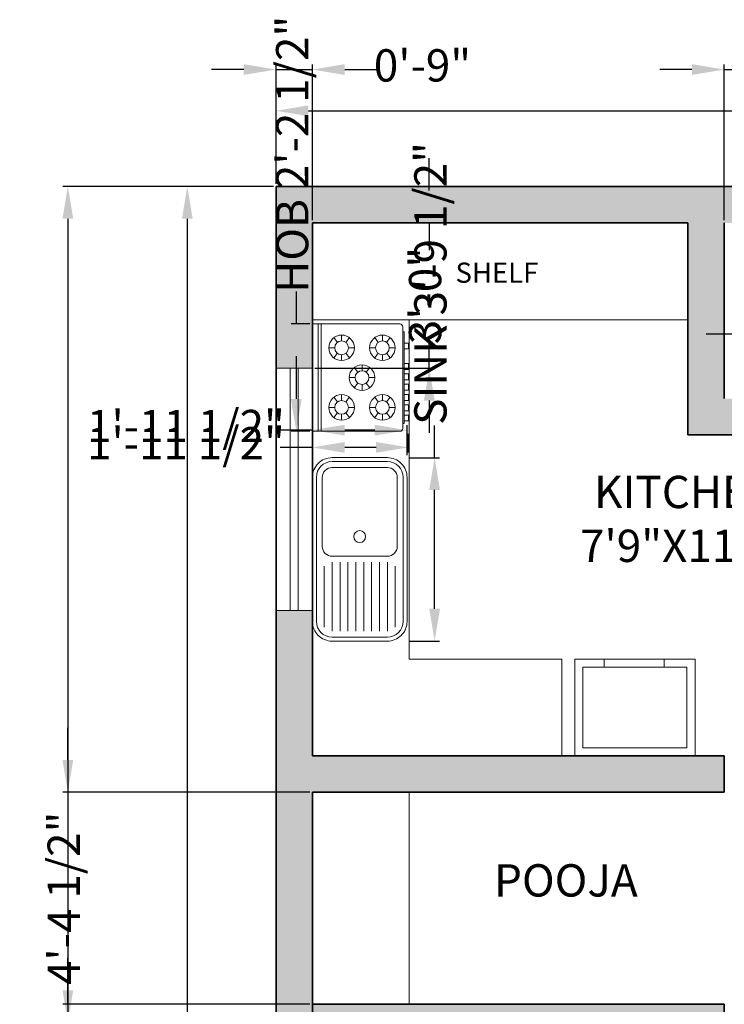
# Model space of a CAD drawing. Units: inches. Extents: x 2408 to 5087, y 2429 to 5085.
# Tile 10 of 12: x 2421 to 2595, y 2815 to 3058. Entities that reach past the tile are written whole.
import ezdxf

# ---------------------------------------------------------------- set-up
doc = ezdxf.new("R2010")
doc.units = ezdxf.units.IN
for name, color, linetype, lineweight in [('A-ANNO-DIMS', 2, 'Continuous', 18), ('A-ANNO-TEXT', 6, 'Continuous', 18), ('A-AREA-IDEN', 6, 'Continuous', 18), ('A-EQPM', 53, 'Continuous', 18), ('A-FLOR-CASE', 8, 'Continuous', 18), ('A-FLOR-FIXT', 9, 'Continuous', 18), ('A-GLAZ', 4, 'Continuous', 18), ('A-WALL', 7, 'Continuous', 35), ('A-WALL-PATT', 252, 'Continuous', 13)]:
    doc.layers.add(name, color=color, linetype=linetype, lineweight=lineweight)
doc.styles.get("Standard").update_dxf_attribs({"font": 'arial.ttf'})
doc.dimstyles.new('ISO-25', dxfattribs={"dimtxt": 8, "dimasz": 8, "dimexe": 1.25, "dimexo": 0.625, "dimtad": 0, "dimdec": 1, "dimlunit": 4, "dimtxsty": 'Standard', "dimcen": 2.5, "dimadec": 0, "dimazin": 0, "dimtfac": 1, "dimtdec": 1, "dimtmove": 0, "dimatfit": 3, "dimfxl": 1, "dimarcsym": 0})

# ---------------------------------------------------------------- blocks, each defined once
blk = doc.blocks.new('*D1')
at = {"layer": 'A-ANNO-DIMS', "color": 0, "lineweight": -2, "transparency": 16777216}
for p, q in [((2484.49, 3017.68), (2484.49, 3037.05)), ((2492.49, 3035.8), (2639.56, 3035.8)), ((2815.49, 3035.8), (2668.43, 3035.8)), ((2823.49, 3017.68), (2823.49, 3037.05))]:
    blk.add_line(p, q, dxfattribs=at)
at = {"layer": 'A-ANNO-DIMS', "color": 0, "transparency": 16777216}
for points in [[(2492.49, 3037.13), (2492.49, 3034.47), (2484.49, 3035.8)], [(2815.49, 3037.13), (2815.49, 3034.47), (2823.49, 3035.8)]]:
    blk.add_solid(points, dxfattribs=at)
at = {"layer": 'Defpoints', "color": 0, "transparency": 16777216}
for p in [(2823.49, 3035.8), (2484.49, 3017.05), (2823.49, 3017.05)]:
    blk.add_point(p, dxfattribs=at)
at = {"layer": 'A-ANNO-DIMS', "color": 0, "transparency": 16777216, "insert": (2653.99, 3035.8), "char_height": 8, "attachment_point": 5}
blk.add_mtext('28\'-3"', dxfattribs=at)
blk = doc.blocks.new('*D2')
at = {"layer": 'A-ANNO-DIMS', "color": 0, "lineweight": -2, "transparency": 16777216}
for p, q in [((2483.87, 3017.05), (2461.26, 3017.05)), ((2462.51, 3009.05), (2462.51, 2772.63)), ((2462.51, 2521.05), (2462.51, 2757.48)), ((2483.87, 2513.05), (2461.26, 2513.05))]:
    blk.add_line(p, q, dxfattribs=at)
at = {"layer": 'A-ANNO-DIMS', "color": 0, "transparency": 16777216}
for points in [[(2461.17, 3009.05), (2463.84, 3009.05), (2462.51, 3017.05)], [(2461.17, 2521.05), (2463.84, 2521.05), (2462.51, 2513.05)]]:
    blk.add_solid(points, dxfattribs=at)
at = {"layer": 'Defpoints', "color": 0, "transparency": 16777216}
for p in [(2484.49, 3017.05), (2462.51, 2513.05), (2484.49, 2513.05)]:
    blk.add_point(p, dxfattribs=at)
at = {"layer": 'A-ANNO-DIMS', "color": 0, "transparency": 16777216, "insert": (2462.51, 2765.05), "char_height": 8, "attachment_point": 5, "rotation": 90}
blk.add_mtext("42'", dxfattribs=at)
blk = doc.blocks.new('g')
for p, q in [((2588.75, 3095.5), (2617.52, 3095.5)), ((2588.75, 3095.5), (2588.75, 3072.07)), ((2617.52, 3095.5), (2617.52, 3072.07)), ((2588.75, 3093.93), (2617.52, 3093.93)), ((2588.75, 3093.14), (2617.52, 3093.14)), ((2593.68, 3088.79), (2592.42, 3089.75)), ((2595.15, 3091.1), (2595.15, 3089.52)), ((2596.62, 3088.79), (2597.87, 3089.75)), ((2609.65, 3088.79), (2608.4, 3089.75)), ((2611.12, 3091.1), (2611.12, 3089.52)), ((2612.59, 3088.79), (2613.85, 3089.75)), ((2593.3, 3087.68), (2591.72, 3087.68)), ((2598.57, 3087.68), (2596.99, 3087.68)), ((2607.7, 3087.68), (2609.28, 3087.68)), ((2612.97, 3087.68), (2614.55, 3087.68)), ((2592.42, 3085.61), (2593.68, 3086.56)), ((2595.15, 3085.83), (2595.15, 3084.25)), ((2597.87, 3085.61), (2596.62, 3086.56)), ((2601.66, 3083.33), (2600.41, 3084.28)), ((2603.14, 3085.64), (2603.14, 3084.06)), ((2604.61, 3083.33), (2605.86, 3084.28)), ((2608.4, 3085.61), (2609.65, 3086.56)), ((2611.12, 3085.83), (2611.12, 3084.25)), ((2613.85, 3085.61), (2612.59, 3086.56)), ((2601.29, 3082.21), (2599.71, 3082.21)), ((2606.56, 3082.21), (2604.98, 3082.21)), ((2592.42, 3078.82), (2593.68, 3077.87)), ((2595.15, 3078.6), (2595.15, 3080.17)), ((2597.87, 3078.82), (2596.62, 3077.87)), ((2600.41, 3080.14), (2601.66, 3081.09)), ((2603.14, 3080.36), (2603.14, 3078.79)), ((2605.86, 3080.14), (2604.61, 3081.09)), ((2608.4, 3078.82), (2609.65, 3077.87)), ((2611.12, 3078.6), (2611.12, 3080.17)), ((2613.85, 3078.82), (2612.59, 3077.87)), ((2593.3, 3076.75), (2591.72, 3076.75)), ((2598.57, 3076.75), (2596.99, 3076.75)), ((2607.7, 3076.75), (2609.28, 3076.75)), ((2612.97, 3076.75), (2614.55, 3076.75)), ((2593.68, 3075.63), (2592.42, 3074.68)), ((2595.15, 3073.33), (2595.15, 3074.9)), ((2596.62, 3075.63), (2597.87, 3074.68)), ((2609.65, 3075.63), (2608.4, 3074.68)), ((2611.12, 3073.33), (2611.12, 3074.9)), ((2612.59, 3075.63), (2613.85, 3074.68)), ((2589.54, 3071.29), (2616.73, 3071.29)), ((2590.84, 3070.89), (2590.84, 3071.29)), ((2590.84, 3070.89), (2615.43, 3070.89)), ((2591.53, 3070.89), (2591.53, 3069.8)), ((2593.12, 3069.8), (2593.12, 3070.89)), ((2594.28, 3070.89), (2594.28, 3069.8)), ((2595.88, 3069.8), (2595.88, 3070.89)), ((2597.04, 3070.89), (2597.04, 3069.8)), ((2598.63, 3069.8), (2598.63, 3070.89)), ((2599.79, 3070.89), (2599.79, 3069.8)), ((2601.39, 3069.8), (2601.39, 3070.89)), ((2602.55, 3070.89), (2602.55, 3069.8)), ((2604.14, 3069.8), (2604.14, 3070.89)), ((2605.31, 3070.89), (2605.31, 3069.8)), ((2606.9, 3069.8), (2606.9, 3070.89)), ((2610.82, 3070.89), (2610.82, 3069.8)), ((2612.41, 3069.8), (2612.41, 3070.89)), ((2615.43, 3070.89), (2615.43, 3071.29)), ((2591.53, 3069.8), (2593.12, 3069.8)), ((2594.28, 3069.8), (2595.88, 3069.8)), ((2597.04, 3069.8), (2598.63, 3069.8)), ((2599.79, 3069.8), (2601.39, 3069.8)), ((2602.55, 3069.8), (2604.14, 3069.8)), ((2605.31, 3069.8), (2606.9, 3069.8)), ((2610.82, 3069.8), (2612.41, 3069.8))]:
    blk.add_line(p, q)
for centre, radius in [((2595.15, 3087.68), 3.42), ((2595.15, 3087.68), 1.85), ((2611.12, 3087.68), 3.42), ((2611.12, 3087.68), 1.85), ((2603.14, 3082.21), 3.42), ((2603.14, 3082.21), 1.85), ((2595.15, 3076.75), 3.42), ((2611.12, 3076.75), 3.42), ((2595.15, 3076.75), 1.85), ((2611.12, 3076.75), 1.85)]:
    blk.add_circle(centre, radius)
for centre, start, end in [((2589.54, 3072.07), 180, 270), ((2616.73, 3072.07), 270, 0)]:
    blk.add_arc(centre, 0.787, start, end)
blk = doc.blocks.new('sink')
for p, q in [((2402.653, 2953.482), (2405.527, 2953.482)), ((2402.535, 2953.325), (2403.755, 2953.325)), ((2402.338, 2952.065), (2402.338, 2953.167)), ((2402.456, 2953.167), (2403.834, 2953.167)), ((2405.842, 2953.167), (2405.842, 2952.065)), ((2402.456, 2953.01), (2403.834, 2953.01)), ((2402.456, 2952.852), (2403.834, 2952.852)), ((2402.456, 2952.695), (2403.834, 2952.695)), ((2402.456, 2952.537), (2403.834, 2952.537)), ((2402.456, 2952.38), (2403.834, 2952.38)), ((2402.456, 2952.222), (2403.834, 2952.222)), ((2402.456, 2952.065), (2403.834, 2952.065)), ((2402.535, 2951.907), (2403.755, 2951.907)), ((2405.527, 2951.75), (2402.653, 2951.75))]:
    blk.add_line(p, q)
at = {"flags": 128}
for points in [[(2405.527, 2953.561, -0.414214), (2405.921, 2953.167), (2405.921, 2952.065, -0.414214), (2405.527, 2951.671), (2402.653, 2951.671, -0.414214), (2402.259, 2952.065), (2402.259, 2953.167, -0.414214), (2402.653, 2953.561)], [(2405.527, 2953.364, -0.414214), (2405.724, 2953.167), (2405.724, 2952.065, -0.414214), (2405.527, 2951.868), (2404.149, 2951.868, -0.414214), (2403.952, 2952.065), (2403.952, 2953.167, -0.414214), (2404.149, 2953.364)]]:
    blk.add_lwpolyline(points, format="xyb", close=True, dxfattribs=at)
blk.add_circle((2404.346, 2952.616), 0.118)
for centre, start, end in [((2402.653, 2953.167), 90, 180), ((2405.527, 2953.167), 0, 90), ((2402.653, 2952.065), 180, 270), ((2405.527, 2952.065), 270, 0)]:
    blk.add_arc(centre, 0.315, start, end)
blk = doc.blocks.new('WIN-60x9')
for p, q in [((3.5, 60), (3.5, 0)), ((5.5, 60), (5.5, 0))]:
    blk.add_line(p, q)
blk.add_lwpolyline([(0, 60), (9, 60), (9, 0), (0, 0)], close=True)
blk = doc.blocks.new('*D48')
at = {"layer": 'A-ANNO-DIMS', "color": 0, "lineweight": -2, "transparency": 16777216}
for p, q in [((2607, 2983.48), (2607, 2979.26)), ((2619.98, 2983.48), (2619.98, 2979.26)), ((2599, 2980.51), (2591, 2980.51)), ((2607, 2980.51), (2619.98, 2980.51)), ((2627.98, 2980.51), (2635.98, 2980.51))]:
    blk.add_line(p, q, dxfattribs=at)
at = {"layer": 'A-ANNO-DIMS', "color": 0, "transparency": 16777216}
for points in [[(2599, 2981.84), (2599, 2979.18), (2607, 2980.51)], [(2627.98, 2981.84), (2627.98, 2979.18), (2619.98, 2980.51)]]:
    blk.add_solid(points, dxfattribs=at)
at = {"layer": 'Defpoints', "color": 0, "transparency": 16777216}
for p in [(2607, 2984.1), (2619.98, 2984.1), (2619.98, 2980.51)]:
    blk.add_point(p, dxfattribs=at)
at = {"layer": 'A-ANNO-DIMS', "color": 0, "transparency": 16777216, "insert": (2660.61, 2980.51), "char_height": 8, "attachment_point": 5}
blk.add_mtext('1\'-1" TYP.', dxfattribs=at)
blk = doc.blocks.new('*D55')
at = {"layer": 'A-ANNO-DIMS', "color": 0, "lineweight": -2, "transparency": 16777216}
for p, q in [((2489.51, 2983.02), (2489.51, 2991.02)), ((2492.87, 2983.02), (2488.26, 2983.02)), ((2489.51, 2964.44), (2489.51, 2975.02)), ((2492.87, 2956.44), (2488.26, 2956.44))]:
    blk.add_line(p, q, dxfattribs=at)
at = {"layer": 'A-ANNO-DIMS', "color": 0, "transparency": 16777216}
for points in [[(2488.17, 2975.02), (2490.84, 2975.02), (2489.51, 2983.02)], [(2488.17, 2964.44), (2490.84, 2964.44), (2489.51, 2956.44)]]:
    blk.add_solid(points, dxfattribs=at)
at = {"layer": 'Defpoints', "color": 0, "transparency": 16777216}
for p in [(2489.51, 2983.02), (2493.49, 2983.02), (2493.49, 2956.44)]:
    blk.add_point(p, dxfattribs=at)
at = {"layer": 'A-ANNO-DIMS', "color": 0, "transparency": 16777216, "insert": (2489.51, 3025.04), "char_height": 8, "attachment_point": 5, "rotation": 90}
blk.add_mtext('HOB 2\'-2 1/2"', dxfattribs=at)
blk = doc.blocks.new('*D56')
at = {"layer": 'A-ANNO-DIMS', "color": 0, "lineweight": -2, "transparency": 16777216}
for p, q in [((2493.49, 2955.81), (2493.49, 2951.2)), ((2517.24, 2955.81), (2517.24, 2951.2)), ((2493.49, 2952.45), (2485.49, 2952.45)), ((2509.24, 2952.45), (2501.49, 2952.45))]:
    blk.add_line(p, q, dxfattribs=at)
at = {"layer": 'A-ANNO-DIMS', "color": 0, "transparency": 16777216}
for points in [[(2501.49, 2953.78), (2501.49, 2951.12), (2493.49, 2952.45)], [(2509.24, 2953.78), (2509.24, 2951.12), (2517.24, 2952.45)]]:
    blk.add_solid(points, dxfattribs=at)
at = {"layer": 'Defpoints', "color": 0, "transparency": 16777216}
for p in [(2493.49, 2956.44), (2517.24, 2956.44), (2493.49, 2952.45)]:
    blk.add_point(p, dxfattribs=at)
at = {"layer": 'A-ANNO-DIMS', "color": 0, "transparency": 16777216, "insert": (2462.18, 2952.45), "char_height": 8, "attachment_point": 5}
blk.add_mtext('1\'-11 1/2"', dxfattribs=at)
blk = doc.blocks.new('*D57')
at = {"layer": 'A-ANNO-DIMS', "color": 0, "lineweight": -2, "transparency": 16777216}
for p, q in [((2523.75, 2949.9), (2523.75, 2957.9)), ((2517.56, 2949.9), (2525, 2949.9)), ((2523.75, 2912.48), (2523.75, 2941.9)), ((2517.56, 2904.48), (2525, 2904.48))]:
    blk.add_line(p, q, dxfattribs=at)
at = {"layer": 'A-ANNO-DIMS', "color": 0, "transparency": 16777216}
for points in [[(2522.42, 2941.9), (2525.08, 2941.9), (2523.75, 2949.9)], [(2522.42, 2912.48), (2525.08, 2912.48), (2523.75, 2904.48)]]:
    blk.add_solid(points, dxfattribs=at)
at = {"layer": 'Defpoints', "color": 0, "transparency": 16777216}
for p in [(2516.94, 2949.9), (2523.75, 2949.9), (2516.94, 2904.48)]:
    blk.add_point(p, dxfattribs=at)
at = {"layer": 'A-ANNO-DIMS', "color": 0, "transparency": 16777216, "insert": (2523.75, 2993.05), "char_height": 8, "attachment_point": 5, "rotation": 90}
blk.add_mtext('SINK 3\'-9 1/2"', dxfattribs=at)
blk = doc.blocks.new('*D58')
at = {"layer": 'A-ANNO-DIMS', "color": 0, "lineweight": -2, "transparency": 16777216}
for p, q in [((2493.49, 2950.53), (2493.49, 2957.96)), ((2516.94, 2950.53), (2516.94, 2957.96)), ((2493.49, 2956.71), (2485.49, 2956.71)), ((2508.94, 2956.71), (2501.49, 2956.71))]:
    blk.add_line(p, q, dxfattribs=at)
at = {"layer": 'A-ANNO-DIMS', "color": 0, "transparency": 16777216}
for points in [[(2501.49, 2958.05), (2501.49, 2955.38), (2493.49, 2956.71)], [(2508.94, 2958.05), (2508.94, 2955.38), (2516.94, 2956.71)]]:
    blk.add_solid(points, dxfattribs=at)
at = {"layer": 'Defpoints', "color": 0, "transparency": 16777216}
for p in [(2493.49, 2956.71), (2493.49, 2949.9), (2516.94, 2949.9)]:
    blk.add_point(p, dxfattribs=at)
at = {"layer": 'A-ANNO-DIMS', "color": 0, "transparency": 16777216, "insert": (2462.18, 2956.71), "char_height": 8, "attachment_point": 5}
blk.add_mtext('1\'-11 1/2"', dxfattribs=at)
blk = doc.blocks.new('*D62')
at = {"layer": 'A-ANNO-DIMS', "color": 0, "lineweight": -2, "transparency": 16777216}
for p, q in [((2432.93, 2875.05), (2432.93, 2883.05)), ((2492.87, 2867.05), (2431.68, 2867.05)), ((2432.93, 2867.05), (2432.93, 2861.54)), ((2432.93, 2814.55), (2432.93, 2820.06)), ((2492.87, 2814.55), (2431.68, 2814.55)), ((2432.93, 2806.55), (2432.93, 2798.55))]:
    blk.add_line(p, q, dxfattribs=at)
at = {"layer": 'A-ANNO-DIMS', "color": 0, "transparency": 16777216}
for points in [[(2431.59, 2875.05), (2434.26, 2875.05), (2432.93, 2867.05)], [(2431.59, 2806.55), (2434.26, 2806.55), (2432.93, 2814.55)]]:
    blk.add_solid(points, dxfattribs=at)
at = {"layer": 'Defpoints', "color": 0, "transparency": 16777216}
for p in [(2432.93, 2867.05), (2493.49, 2867.05), (2493.49, 2814.55)]:
    blk.add_point(p, dxfattribs=at)
at = {"layer": 'A-ANNO-DIMS', "color": 0, "transparency": 16777216, "insert": (2432.93, 2840.8), "char_height": 8, "attachment_point": 5, "rotation": 90}
blk.add_mtext('4\'-4 1/2"', dxfattribs=at)
blk = doc.blocks.new('*D63')
at = {"layer": 'A-ANNO-DIMS', "color": 0, "lineweight": -2, "transparency": 16777216}
for p, q in [((2476.49, 3046), (2468.49, 3046)), ((2484.49, 3017.68), (2484.49, 3047.25)), ((2484.49, 3046), (2493.49, 3046)), ((2493.49, 3008.68), (2493.49, 3047.25)), ((2501.49, 3046), (2509.49, 3046))]:
    blk.add_line(p, q, dxfattribs=at)
at = {"layer": 'A-ANNO-DIMS', "color": 0, "transparency": 16777216}
for points in [[(2476.49, 3047.34), (2476.49, 3044.67), (2484.49, 3046)], [(2501.49, 3047.34), (2501.49, 3044.67), (2493.49, 3046)]]:
    blk.add_solid(points, dxfattribs=at)
at = {"layer": 'Defpoints', "color": 0, "transparency": 16777216}
for p in [(2493.49, 3046), (2484.49, 3017.05), (2493.49, 3008.05)]:
    blk.add_point(p, dxfattribs=at)
at = {"layer": 'A-ANNO-DIMS', "color": 0, "transparency": 16777216, "insert": (2520.75, 3046), "char_height": 8, "attachment_point": 5}
blk.add_mtext('0\'-9"', dxfattribs=at)
blk = doc.blocks.new('*D66')
at = {"layer": 'A-ANNO-DIMS', "color": 0, "lineweight": -2, "transparency": 16777216}
for p, q in [((2483.87, 3017.05), (2431.68, 3017.05)), ((2432.93, 3009.05), (2432.93, 2767.25)), ((2432.93, 2477.75), (2432.93, 2719.56)), ((2461.25, 2469.75), (2431.68, 2469.75))]:
    blk.add_line(p, q, dxfattribs=at)
at = {"layer": 'A-ANNO-DIMS', "color": 0, "transparency": 16777216}
for points in [[(2431.59, 3009.05), (2434.26, 3009.05), (2432.93, 3017.05)], [(2431.59, 2477.75), (2434.26, 2477.75), (2432.93, 2469.75)]]:
    blk.add_solid(points, dxfattribs=at)
at = {"layer": 'Defpoints', "color": 0, "transparency": 16777216}
for p in [(2432.93, 3017.05), (2484.49, 3017.05), (2461.88, 2469.75)]:
    blk.add_point(p, dxfattribs=at)
at = {"layer": 'A-ANNO-DIMS', "color": 0, "transparency": 16777216, "insert": (2432.93, 2743.4), "char_height": 8, "attachment_point": 5, "rotation": 90}
blk.add_mtext('45\'-7 1/2"', dxfattribs=at)
blk = doc.blocks.new('*D70')
at = {"layer": 'A-ANNO-DIMS', "color": 0, "lineweight": -2, "transparency": 16777216}
for p, q in [((2587.49, 3046), (2579.49, 3046)), ((2595.49, 3008.68), (2595.49, 3047.25)), ((2595.49, 3046), (2601.49, 3046)), ((2601.49, 3008.68), (2601.49, 3047.25)), ((2609.49, 3046), (2617.49, 3046))]:
    blk.add_line(p, q, dxfattribs=at)
at = {"layer": 'A-ANNO-DIMS', "color": 0, "transparency": 16777216}
for points in [[(2587.49, 3047.34), (2587.49, 3044.67), (2595.49, 3046)], [(2609.49, 3047.34), (2609.49, 3044.67), (2601.49, 3046)]]:
    blk.add_solid(points, dxfattribs=at)
at = {"layer": 'Defpoints', "color": 0, "transparency": 16777216}
for p in [(2601.49, 3046), (2595.49, 3008.05), (2601.49, 3008.05)]:
    blk.add_point(p, dxfattribs=at)
at = {"layer": 'A-ANNO-DIMS', "color": 0, "transparency": 16777216, "insert": (2628.75, 3046), "char_height": 8, "attachment_point": 5}
blk.add_mtext('0\'-6"', dxfattribs=at)
blk = doc.blocks.new('*D72')
at = {"layer": 'A-ANNO-DIMS', "color": 0, "lineweight": -2, "transparency": 16777216}
for p, q in [((2522.44, 3016.05), (2522.44, 3024.05)), ((2494.12, 3008.05), (2523.69, 3008.05)), ((2522.44, 3008.05), (2522.44, 3001.31)), ((2522.44, 2972.05), (2522.44, 2978.8)), ((2494.12, 2972.05), (2523.69, 2972.05)), ((2522.44, 2964.05), (2522.44, 2956.05))]:
    blk.add_line(p, q, dxfattribs=at)
at = {"layer": 'A-ANNO-DIMS', "color": 0, "transparency": 16777216}
for points in [[(2521.11, 3016.05), (2523.78, 3016.05), (2522.44, 3008.05)], [(2521.11, 2964.05), (2523.78, 2964.05), (2522.44, 2972.05)]]:
    blk.add_solid(points, dxfattribs=at)
at = {"layer": 'Defpoints', "color": 0, "transparency": 16777216}
for p in [(2493.49, 3008.05), (2493.49, 2972.05), (2522.44, 2972.05)]:
    blk.add_point(p, dxfattribs=at)
at = {"layer": 'A-ANNO-DIMS', "color": 0, "transparency": 16777216, "insert": (2522.44, 2990.05), "char_height": 8, "attachment_point": 5, "rotation": 90}
blk.add_mtext('3\'-0"', dxfattribs=at)
blk = doc.blocks.new('*D79')
at = {"layer": 'A-ANNO-DIMS', "color": 0, "lineweight": -2, "transparency": 16777216}
for p, q in [((2432.93, 2818.05), (2432.93, 2826.05)), ((2693.87, 2810.05), (2431.68, 2810.05)), ((2432.93, 2810.05), (2432.93, 2809.38)), ((2432.93, 2786.05), (2432.93, 2786.73)), ((2693.87, 2786.05), (2431.68, 2786.05)), ((2432.93, 2778.05), (2432.93, 2770.05))]:
    blk.add_line(p, q, dxfattribs=at)
at = {"layer": 'A-ANNO-DIMS', "color": 0, "transparency": 16777216}
for points in [[(2431.59, 2818.05), (2434.26, 2818.05), (2432.93, 2810.05)], [(2431.59, 2778.05), (2434.26, 2778.05), (2432.93, 2786.05)]]:
    blk.add_solid(points, dxfattribs=at)
at = {"layer": 'Defpoints', "color": 0, "transparency": 16777216}
for p in [(2432.93, 2810.05), (2694.49, 2810.05), (2694.49, 2786.05)]:
    blk.add_point(p, dxfattribs=at)
at = {"layer": 'A-ANNO-DIMS', "color": 0, "transparency": 16777216, "insert": (2432.93, 2798.05), "char_height": 8, "attachment_point": 5, "rotation": 90}
blk.add_mtext('2\'-0"', dxfattribs=at)

msp = doc.modelspace()

# ---------------------------------------------------------------- hatches: boundary and pattern name
at = {"layer": 'A-WALL-PATT'}
h = msp.add_hatch(color=256, dxfattribs=at)
h.dxf.hatch_style = 1
h.paths.add_polyline_path([(2493.49, 2613.55), (2523.49, 2613.55), (2523.49, 2622.55), (2493.49, 2622.55), (2493.49, 2714.8), (2484.49, 2714.8), (2484.49, 2497.75), (2493.49, 2497.75)])
h.paths.add_polyline_path([(2613.49, 2615.42), (2613.49, 2622.55), (2583.49, 2622.55), (2583.49, 2613.55), (2613.46, 2613.55, -0.009707)])
h.paths.add_polyline_path([(2823.49, 2634.55), (2814.49, 2634.55), (2814.49, 2622.55), (2694.49, 2622.55), (2694.49, 2670.55), (2706.49, 2670.55), (2706.49, 2675.05), (2694.49, 2675.05), (2694.49, 2750.05), (2685.49, 2750.05), (2685.49, 2622.55), (2661.49, 2622.55), (2661.49, 2613.55), (2814.49, 2613.55), (2814.49, 2522.05), (2688.49, 2522.05), (2688.49, 2513.05), (2823.49, 2513.05)])
h.paths.add_polyline_path([(2823.49, 2837.05), (2814.49, 2837.05), (2814.49, 2819.05), (2685.49, 2819.05), (2685.49, 2786.05), (2694.49, 2786.05), (2694.49, 2810.05), (2814.49, 2810.05), (2814.49, 2772.55), (2823.49, 2772.55)])
h.paths.add_polyline_path([(2694.49, 2964.55), (2595.49, 2964.55), (2595.49, 3008.05), (2601.49, 3008.05), (2601.49, 3017.05), (2484.49, 3017.05), (2484.49, 2972.05), (2493.49, 2972.05), (2493.49, 3008.05), (2586.49, 3008.05), (2586.49, 2955.55), (2685.49, 2955.55), (2685.49, 2854.87), (2694.49, 2854.87)])
h.paths.add_polyline_path([(2493.49, 2867.05), (2595.49, 2867.05), (2595.49, 2876.05), (2493.49, 2876.05), (2493.49, 2912.05), (2484.49, 2912.05), (2484.49, 2774.8), (2493.49, 2774.8)])
h.paths.add_polyline_path([(2595.49, 2814.55), (2493.49, 2814.55), (2493.49, 2810.05), (2595.49, 2810.05)], flags=17)
h.paths.add_polyline_path([(2724.49, 3017.05), (2625.49, 3017.05), (2625.49, 3008.05), (2685.49, 3008.05), (2685.49, 2994.55), (2694.49, 2994.55), (2694.49, 3008.05), (2724.49, 3008.05)])
h.paths.add_polyline_path([(2823.49, 3017.05), (2784.49, 3017.05), (2784.49, 3008.05), (2814.49, 3008.05), (2814.49, 2913.55), (2814.56, 2897.05), (2823.49, 2897.05)])
h.paths.add_polyline_path([(2823.49, 2712.55), (2814.61, 2712.55), (2814.66, 2701.27), (2814.49, 2701.27), (2814.49, 2675.05), (2740.99, 2675.05), (2740.99, 2687.05), (2736.49, 2687.05), (2736.49, 2670.55), (2814.49, 2670.55), (2814.49, 2658.55), (2823.49, 2658.55)], flags=17)

# ---------------------------------------------------------------- linework, layer by layer
at = {"layer": 'A-EQPM'}
for p, q in [((2588.25, 2900.05), (2558.48, 2900.05)), ((2565.77, 2898.05), (2565.77, 2900.05)), ((2580.63, 2898.05), (2580.63, 2900.05)), ((2588.25, 2900.05), (2588.25, 2876.05))]:
    msp.add_line(p, q, dxfattribs=at)
for points in [[(2588.25, 2876.05), (2558.48, 2876.05), (2558.48, 2900.05), (2588.25, 2900.05)], [(2586.25, 2878.05), (2560.48, 2878.05), (2560.48, 2898.05), (2586.25, 2898.05)]]:
    msp.add_lwpolyline(points, close=True, dxfattribs=at)
at = {"layer": 'A-FLOR-CASE'}
for p, q in [((2586.49, 2984.05), (2493.49, 2984.05)), ((2517.49, 2984.05), (2517.49, 2900.05)), ((2555.29, 2900.05), (2517.49, 2900.05)), ((2555.29, 2900.05), (2555.29, 2876.05)), ((2517.49, 2867.05), (2517.49, 2814.55))]:
    msp.add_line(p, q, dxfattribs=at)
at = {"layer": 'A-WALL'}
for p, q in [((2823.49, 3017.05), (2484.49, 3017.05)), ((2484.49, 3017.05), (2484.49, 2497.75)), ((2493.49, 3008.05), (2493.49, 2876.05)), ((2586.49, 3008.05), (2493.49, 3008.05)), ((2586.49, 3008.05), (2586.49, 2955.55)), ((2595.49, 3008.05), (2595.49, 2964.55)), ((2685.49, 2955.55), (2586.49, 2955.55)), ((2595.49, 2876.05), (2493.49, 2876.05)), ((2595.49, 2876.05), (2595.49, 2867.05)), ((2595.49, 2867.05), (2493.49, 2867.05)), ((2493.49, 2867.05), (2493.49, 2622.55)), ((2595.49, 2814.55), (2493.49, 2814.55)), ((2595.49, 2814.55), (2595.49, 2810.05))]:
    msp.add_line(p, q, dxfattribs=at)

# ---------------------------------------------------------------- block references
at = {"layer": 'A-EQPM', "xscale": 0.9241143459422847, "yscale": 0.9241143459422847, "zscale": 0.9241143459422847, "rotation": 90}
msp.add_blockref('g', (5354.09, 564.13), dxfattribs=at)
at = {"layer": 'A-FLOR-FIXT', "xscale": 12.40512744421288, "yscale": 12.40512744421288, "zscale": 12.40512744421288, "rotation": 90}
msp.add_blockref('sink', (39132.79, -26895.85), dxfattribs=at)
at = {"layer": 'A-GLAZ'}
msp.add_blockref('WIN-60x9', (2484.49, 2912.05), dxfattribs=at)

# ---------------------------------------------------------------- texts
at = {"layer": 'A-ANNO-TEXT', "insert": (2487.74, 2998.21), "char_height": 5, "attachment_point": 1}
msp.add_mtext_dynamic_manual_height_columns('\\pxqc;SHELF', width=102.8772, gutter_width=12.5, heights=[0], dxfattribs=at)
at = {"layer": 'A-AREA-IDEN', "char_height": 8, "attachment_point": 1}
for s, insert in [('\\pxqc;KITCHEN\\P7\'9"X11\'0"', (2534.8, 2945.41)), ('\\pxqc;POOJA', (2504.82, 2849.24))]:
    msp.add_mtext_dynamic_manual_height_columns(s, width=102.8772, gutter_width=12.5, heights=[0], dxfattribs=dict(at, insert=insert))

# ---------------------------------------------------------------- dimensions: what is measured, and where the dimension line sits
at = {"layer": 'A-ANNO-DIMS'}
for base, p1, p2, text, picture, middle in [((2489.51, 2983.02), (2493.49, 2956.44), (2493.49, 2983.02), 'HOB <>', '*D55', (2489.51, 3025.04)), ((2523.75, 2949.9), (2516.94, 2904.48), (2516.94, 2949.9), 'SINK <>', '*D57', (2523.75, 2993.05))]:
    dim = msp.add_linear_dim(base=base, p1=p1, p2=p2, angle=90, text=text, dimstyle='ISO-25', override={"dimdec": 1, "dimlfac": 1, "dimrnd": 0, "dimzin": 1, "dimdsep": 46, "dimlunit": 4, "dimfrac": 2}, dxfattribs=at)
    dim.commit()
    dim.dimension.update_dxf_attribs({"geometry": picture, "text_midpoint": middle})
for base, p1, p2, override, picture, middle in [((2493.49, 3046), (2484.49, 3017.05), (2493.49, 3008.05), {"dimdec": 1, "dimlfac": 1, "dimrnd": 0, "dimzin": 1, "dimdsep": 46, "dimlunit": 4, "dimfrac": 2}, '*D63', (2520.75, 3046)), ((2601.49, 3046), (2595.49, 3008.05), (2601.49, 3008.05), {"dimdec": 1, "dimlfac": 1, "dimrnd": 0, "dimzin": 1, "dimdsep": 46, "dimlunit": 4, "dimfrac": 2}, '*D70', (2628.75, 3046)), ((2823.49, 3035.8), (2484.49, 3017.05), (2823.49, 3017.05), {"dimclrd": 0, "dimclre": 0, "dimclrt": 0}, '*D1', (2653.99, 3035.8))]:
    dim = msp.add_linear_dim(base=base, p1=p1, p2=p2, dimstyle='ISO-25', override=override, dxfattribs=at)
    dim.commit()
    dim.dimension.update_dxf_attribs({"geometry": picture, "text_midpoint": middle})
for base, p1, p2, angle, override, picture, middle in [((2522.44, 2972.05), (2493.49, 3008.05), (2493.49, 2972.05), 270, {"dimdec": 1, "dimlfac": 1, "dimrnd": 0, "dimzin": 1, "dimdsep": 46, "dimlunit": 4, "dimfrac": 2}, '*D72', (2522.44, 2990.05)), ((2432.93, 3017.05), (2461.88, 2469.75), (2484.49, 3017.05), 90, {"dimdec": 1, "dimlfac": 1, "dimrnd": 0, "dimzin": 1, "dimdsep": 46, "dimlunit": 4, "dimfrac": 2}, '*D66', (2432.93, 2743.4)), ((2462.51, 2513.05), (2484.49, 3017.05), (2484.49, 2513.05), 90, {"dimclrd": 0, "dimclre": 0, "dimclrt": 0}, '*D2', (2462.51, 2765.05)), ((2493.4939, 2956.7136), (2516.9366, 2949.9005), (2493.4939, 2949.9005), 180, {"dimdec": 1, "dimlfac": 1, "dimrnd": 0, "dimzin": 1, "dimdsep": 46, "dimlunit": 4, "dimfrac": 2}, '*D58', (2462.184, 2956.7136)), ((2493.4939, 2952.4512), (2517.2425, 2956.438), (2493.4939, 2956.438), 180, {"dimdec": 1, "dimlfac": 1, "dimrnd": 0, "dimzin": 1, "dimdsep": 46, "dimlunit": 4, "dimfrac": 2}, '*D56', (2462.184, 2952.4512)), ((2432.93, 2867.05), (2493.49, 2814.55), (2493.49, 2867.05), 90, {"dimdec": 1, "dimlfac": 1, "dimrnd": 0, "dimzin": 1, "dimdsep": 46, "dimlunit": 4, "dimfrac": 2}, '*D62', (2432.93, 2840.8)), ((2432.93, 2810.05), (2694.49, 2786.05), (2694.49, 2810.05), 90, {"dimdec": 1, "dimlfac": 1, "dimrnd": 0, "dimzin": 1, "dimdsep": 46, "dimlunit": 4, "dimfrac": 2}, '*D79', (2432.93, 2798.05))]:
    dim = msp.add_linear_dim(base=base, p1=p1, p2=p2, angle=angle, dimstyle='ISO-25', override=override, dxfattribs=at)
    dim.commit()
    dim.dimension.update_dxf_attribs({"geometry": picture, "text_midpoint": middle})
dim = msp.add_linear_dim(base=(2619.98, 2980.51), p1=(2607, 2984.1), p2=(2619.98, 2984.1), text='<> TYP.', dimstyle='ISO-25', override={"dimdec": 1, "dimlfac": 1, "dimrnd": 0, "dimzin": 1, "dimdsep": 46, "dimlunit": 4, "dimfrac": 2}, dxfattribs=at)
dim.commit()
dim.dimension.update_dxf_attribs({"geometry": '*D48', "text_midpoint": (2660.61, 2980.51)})

doc.saveas('drawing.dxf')
